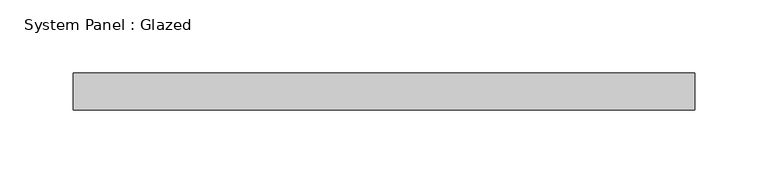
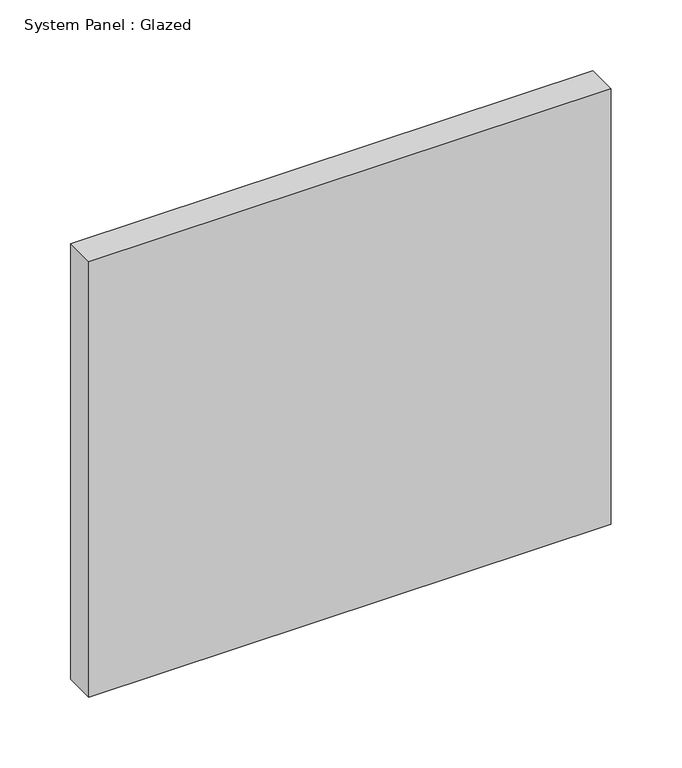
"""IFC4 building model written with IfcOpenShell, lengths in millimetres: plate geometry, System Panel : Glazed."""

from ifc_helpers import new_model, si_unit, origin, origin_with_axes, place, context, project, spatial, polyline, outline, extrude, source, transform, mapped, element, save


def system_panel_glazed_6ee44b12(model_context):
    return source(origin(), model_context, "Body", "SweptSolid", [
        extrude(outline(polyline([(212.725, 19.05), (-212.725, 19.05), (-212.725, 44.45), (212.725, 44.45), (212.725, 19.05)])), origin_with_axes(), (0.0, 0.0, 1.0), 374.65),
    ])


if __name__ == "__main__":
    model = new_model("IFC4")
    model_context = context("Model", 3, world=origin())
    ifc_project = project(units=[si_unit("LENGTHUNIT", "METRE", prefix="MILLI")], contexts=[model_context])
    site = spatial("IfcSite", under=ifc_project)
    building = spatial("IfcBuilding", under=site)
    placement = place(None, origin())
    system_panel_glazed_shape = system_panel_glazed_6ee44b12(model_context)
    element("IfcPlate", 1, ObjectType="System Panel : Glazed", at=placement, inside=building, context=model_context, shape_type="MappedRepresentation", body=[
        mapped(system_panel_glazed_shape, transform((0.0, 0.0, 0.0), x_axis=(1.0, 0.0, 0.0), y_axis=(0.0, 1.0, 0.0), z_axis=(0.0, 0.0, 1.0))),
    ])
    save(model, "model.ifc")

# Revit data of these elements
# Type "System Panel : Glazed"
#   Construction Type Id = "GSP4R"
#   Analytic Construction = "1/8 in Pilkington single glazing"
#   Visual Light Transmittance = 0.9
#   Solar Heat Gain Coefficient = 0.86
#   Heat Transfer Coefficient (U) = 1.18115 BTU/(h·ft²·°F)
#   Define Thermal Properties by = 1
# Element 1 (IfcPlate, "System Panel : Glazed")
#   Materials on its faces: "Glass"
# Materials
#   "Glass": class "Glass", colour RGB 0 128 192, transparency 0.75, Description = "Soda Lime Glass", Cost = 0
